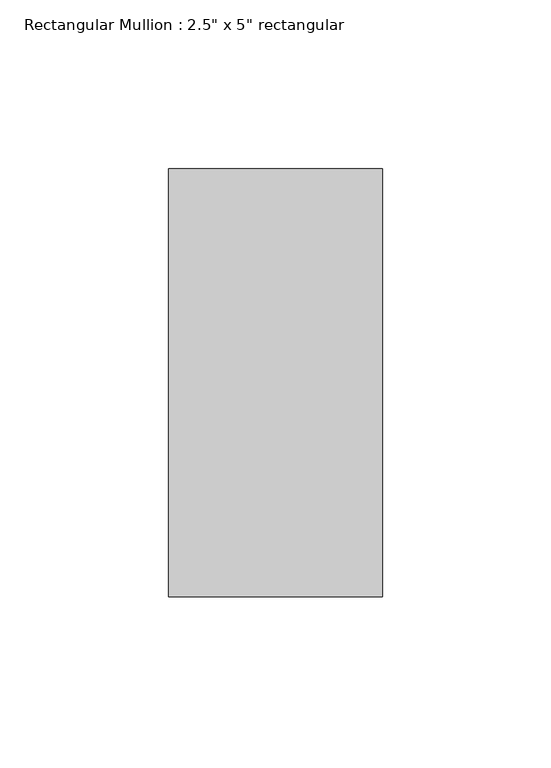
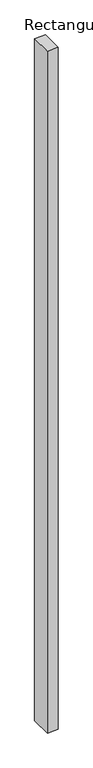
"""IFC4 building model written with IfcOpenShell, lengths in millimetres: member geometry."""

from ifc_helpers import new_model, si_unit, frame, origin, place, context, project, spatial, polyline, outline, extrude, source, transform, mapped, element, save


def member_d965e02f(model_context):
    return source(origin(), model_context, "Body", "SweptSolid", [
        extrude(outline(polyline([(0.0, 63.5), (0.0, -63.5), (-63.5, -63.5), (-63.5, 63.5), (0.0, 63.5)])), frame((0.0, 0.0, -4183.7935364), z_axis=(0.0, 0.0, 1.0), x_axis=(1.0, 0.0, 0.0)), (0.0, 0.0, 1.0), 4183.7935364),
    ])


if __name__ == "__main__":
    model = new_model("IFC4")
    model_context = context("Model", 3, world=origin())
    ifc_project = project(units=[si_unit("LENGTHUNIT", "METRE", prefix="MILLI")], contexts=[model_context])
    site = spatial("IfcSite", under=ifc_project)
    building = spatial("IfcBuilding", under=site)
    placement = place(None, origin())
    member_shape = member_d965e02f(model_context)
    element("IfcMember", 1, ObjectType="Rectangular Mullion : 2.5\" x 5\" rectangular", at=placement, inside=building, context=model_context, shape_type="MappedRepresentation", body=[
        mapped(member_shape, transform((0.0, 0.0, 0.0), x_axis=(1.0, 0.0, 0.0), y_axis=(0.0, 1.0, 0.0), z_axis=(0.0, 0.0, 1.0))),
    ])
    save(model, "model.ifc")

# Revit data of these elements
# Type "Rectangular Mullion : 2.5\" x 5\" rectangular"
#   built-in parameter 1007304 = 0.416667 (stored number, unit not read)
#   built-in parameter 1007301 = 0.104167 (stored number, unit not read)
#   built-in parameter 1007300 = 0.104167 (stored number, unit not read)
# Element 1 (IfcMember, "Rectangular Mullion : 2.5\" x 5\" rectangular")
#   Materials on its faces: "Aluminum"
# Materials
#   "Aluminum": class "Metal", colour RGB 247 247 247, transparency 0, Description = "Aluminum 6061", Cost = 0
